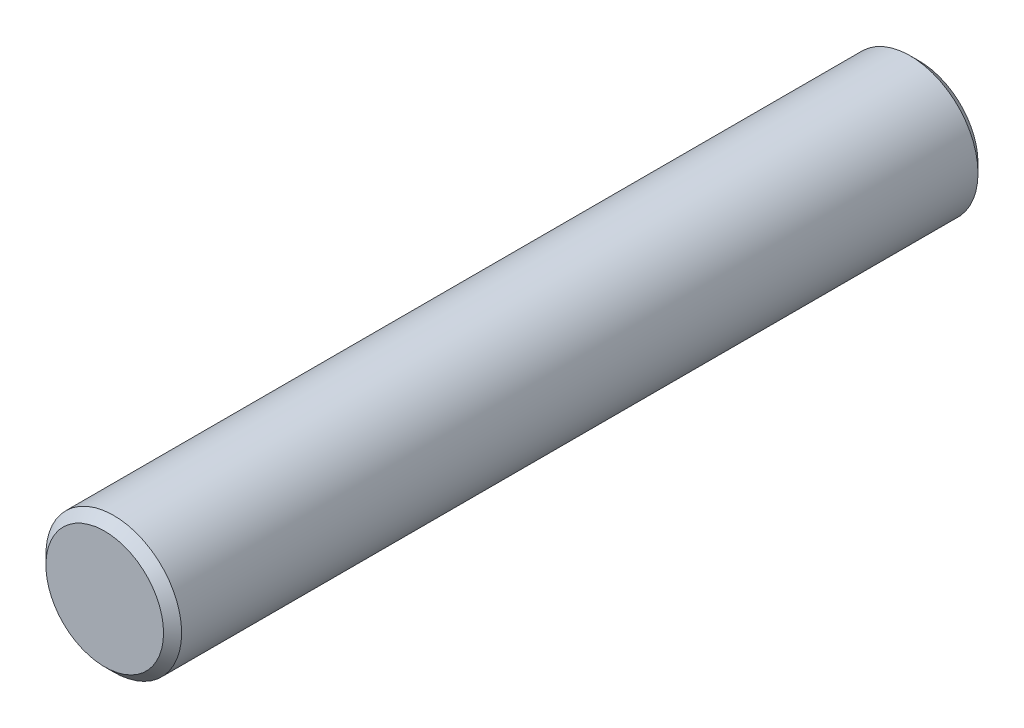
ISO-10303-21;
HEADER;
FILE_DESCRIPTION(('STEP AP214'),'2;1');
FILE_NAME('part.step','',(''),(''),'','','');
FILE_SCHEMA(('AUTOMOTIVE_DESIGN { 1 0 10303 214 1 1 1 1 }'));
ENDSEC;
DATA;
#1=APPLICATION_CONTEXT('core data for automotive mechanical design processes');
#2=APPLICATION_PROTOCOL_DEFINITION('international standard','automotive_design',2000,#1);
#3=PRODUCT_CONTEXT('',#1,'mechanical');
#4=PRODUCT('Part','Part','',(#3));
#5=PRODUCT_RELATED_PRODUCT_CATEGORY('part','',(#4));
#6=PRODUCT_DEFINITION_FORMATION('','',#4);
#7=PRODUCT_DEFINITION_CONTEXT('part definition',#1,'design');
#8=PRODUCT_DEFINITION('design','',#6,#7);
#9=PRODUCT_DEFINITION_SHAPE('','',#8);
#10=(LENGTH_UNIT() NAMED_UNIT(*) SI_UNIT(.MILLI.,.METRE.));
#11=(NAMED_UNIT(*) PLANE_ANGLE_UNIT() SI_UNIT($,.RADIAN.));
#12=(NAMED_UNIT(*) SI_UNIT($,.STERADIAN.) SOLID_ANGLE_UNIT());
#13=UNCERTAINTY_MEASURE_WITH_UNIT(LENGTH_MEASURE(1.E-05),#10,'distance_accuracy_value','');
#14=(GEOMETRIC_REPRESENTATION_CONTEXT(3) GLOBAL_UNCERTAINTY_ASSIGNED_CONTEXT((#13)) GLOBAL_UNIT_ASSIGNED_CONTEXT((#10,
#11,#12)) REPRESENTATION_CONTEXT('',''));
#15=CARTESIAN_POINT('',(0.,0.,0.));
#16=DIRECTION('',(0.,0.,1.));
#17=DIRECTION('',(1.,0.,0.));
#18=AXIS2_PLACEMENT_3D('',#15,#16,#17);
#19=CARTESIAN_POINT('',(0.,0.,9.));
#20=DIRECTION('',(0.,0.,-1.));
#21=DIRECTION('',(-1.,0.,0.));
#22=AXIS2_PLACEMENT_3D('',#19,#20,#21);
#23=CYLINDRICAL_SURFACE('',#22,1.5);
#24=CARTESIAN_POINT('',(0.,0.,8.8));
#25=DIRECTION('',(0.,0.,1.));
#26=DIRECTION('',(1.,0.,0.));
#27=AXIS2_PLACEMENT_3D('',#24,#25,#26);
#28=CIRCLE('',#27,1.5);
#29=CARTESIAN_POINT('',(1.5,0.,8.8));
#30=VERTEX_POINT('',#29);
#31=EDGE_CURVE('E50',#30,#30,#28,.F.);
#32=ORIENTED_EDGE('',*,*,#31,.T.);
#33=EDGE_LOOP('',(#32));
#34=FACE_BOUND('',#33,.T.);
#35=CARTESIAN_POINT('',(0.,0.,-8.8));
#36=DIRECTION('',(0.,0.,1.));
#37=DIRECTION('',(1.,0.,0.));
#38=AXIS2_PLACEMENT_3D('',#35,#36,#37);
#39=CIRCLE('',#38,1.5);
#40=CARTESIAN_POINT('',(1.5,0.,-8.8));
#41=VERTEX_POINT('',#40);
#42=EDGE_CURVE('E51',#41,#41,#39,.T.);
#43=ORIENTED_EDGE('',*,*,#42,.T.);
#44=EDGE_LOOP('',(#43));
#45=FACE_BOUND('',#44,.T.);
#46=ADVANCED_FACE('F39',(#34,#45),#23,.T.);
#47=CARTESIAN_POINT('',(0.,0.,9.));
#48=DIRECTION('',(0.,0.,1.));
#49=DIRECTION('',(1.,0.,0.));
#50=AXIS2_PLACEMENT_3D('',#47,#48,#49);
#51=PLANE('',#50);
#52=CARTESIAN_POINT('',(0.,0.,9.));
#53=DIRECTION('',(0.,0.,1.));
#54=DIRECTION('',(1.,0.,0.));
#55=AXIS2_PLACEMENT_3D('',#52,#53,#54);
#56=CIRCLE('',#55,1.3);
#57=CARTESIAN_POINT('',(1.3,0.,9.));
#58=VERTEX_POINT('',#57);
#59=EDGE_CURVE('E54',#58,#58,#56,.T.);
#60=ORIENTED_EDGE('',*,*,#59,.T.);
#61=EDGE_LOOP('',(#60));
#62=FACE_BOUND('',#61,.T.);
#63=ADVANCED_FACE('F64',(#62),#51,.T.);
#64=CARTESIAN_POINT('',(0.,0.,-9.));
#65=DIRECTION('',(0.,0.,1.));
#66=DIRECTION('',(1.,0.,0.));
#67=AXIS2_PLACEMENT_3D('',#64,#65,#66);
#68=PLANE('',#67);
#69=CARTESIAN_POINT('',(0.,0.,-9.));
#70=DIRECTION('',(0.,0.,1.));
#71=DIRECTION('',(1.,0.,0.));
#72=AXIS2_PLACEMENT_3D('',#69,#70,#71);
#73=CIRCLE('',#72,1.3);
#74=CARTESIAN_POINT('',(1.3,0.,-9.));
#75=VERTEX_POINT('',#74);
#76=EDGE_CURVE('E10',#75,#75,#73,.F.);
#77=ORIENTED_EDGE('',*,*,#76,.T.);
#78=EDGE_LOOP('',(#77));
#79=FACE_BOUND('',#78,.T.);
#80=ADVANCED_FACE('F62',(#79),#68,.F.);
#81=CARTESIAN_POINT('',(0.,0.,9.));
#82=DIRECTION('',(0.,0.,-1.));
#83=DIRECTION('',(-1.,0.,0.));
#84=AXIS2_PLACEMENT_3D('',#81,#82,#83);
#85=CONICAL_SURFACE('',#84,1.3,0.78539816339745);
#86=ORIENTED_EDGE('',*,*,#31,.F.);
#87=EDGE_LOOP('',(#86));
#88=FACE_BOUND('',#87,.T.);
#89=ORIENTED_EDGE('',*,*,#59,.F.);
#90=EDGE_LOOP('',(#89));
#91=FACE_BOUND('',#90,.T.);
#92=ADVANCED_FACE('F65',(#88,#91),#85,.T.);
#93=CARTESIAN_POINT('',(0.,0.,-8.8));
#94=DIRECTION('',(0.,0.,1.));
#95=DIRECTION('',(1.,0.,0.));
#96=AXIS2_PLACEMENT_3D('',#93,#94,#95);
#97=CONICAL_SURFACE('',#96,1.5,0.785398163397446);
#98=ORIENTED_EDGE('',*,*,#76,.F.);
#99=EDGE_LOOP('',(#98));
#100=FACE_BOUND('',#99,.T.);
#101=ORIENTED_EDGE('',*,*,#42,.F.);
#102=EDGE_LOOP('',(#101));
#103=FACE_BOUND('',#102,.T.);
#104=ADVANCED_FACE('F45',(#100,#103),#97,.T.);
#105=CLOSED_SHELL('',(#46,#63,#80,#92,#104));
#106=MANIFOLD_SOLID_BREP('B2',#105);
#107=ADVANCED_BREP_SHAPE_REPRESENTATION('',(#18,#106),#14);
#108=SHAPE_DEFINITION_REPRESENTATION(#9,#107);
ENDSEC;
END-ISO-10303-21;
